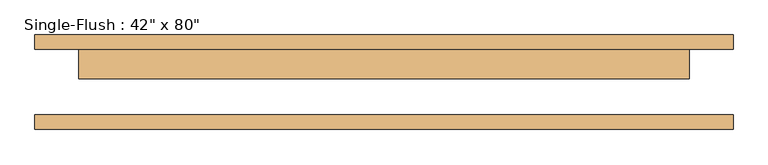
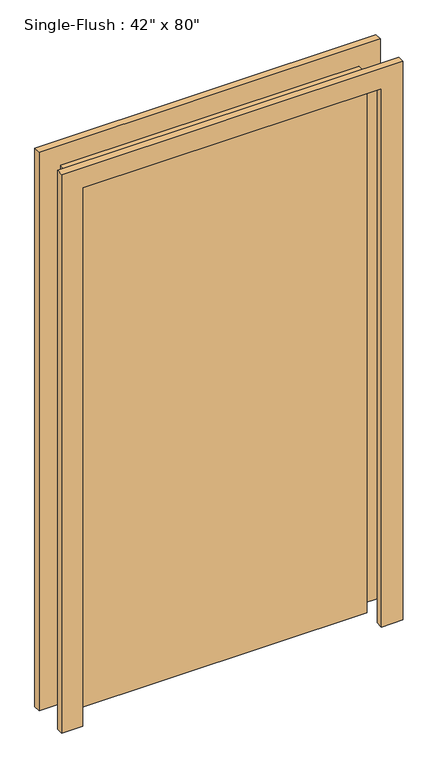
"""IFC4 building model written with IfcOpenShell, lengths in millimetres: door geometry."""

from ifc_helpers import new_model, si_unit, frame, origin, origin_with_axes, place, context, project, spatial, polyline, outline, extrude, source, transform, mapped, element, save


def door_5f0ed9dd(model_context):
    return source(origin(), model_context, "Body", "SweptSolid", [
        extrude(outline(polyline([(2108.2, -609.6), (0.0, -609.6), (0.0, -533.4), (2032.0, -533.4), (2032.0, 533.4), (0.0, 533.4), (0.0, 609.6), (2108.2, 609.6), (2108.2, -609.6)])), frame((0.0, 57.15, 0.0), z_axis=(0.0, 1.0, 0.0), x_axis=(0.0, 0.0, 1.0)), (0.0, 0.0, 1.0), 25.4),
        extrude(outline(polyline([(2108.2, 609.6), (2108.2, -609.6), (0.0, -609.6), (0.0, -533.4), (2032.0, -533.4), (2032.0, 533.4), (0.0, 533.4), (0.0, 609.6), (2108.2, 609.6)])), frame((0.0, -82.55, 0.0), z_axis=(0.0, 1.0, 0.0), x_axis=(0.0, 0.0, 1.0)), (0.0, 0.0, 1.0), 25.4),
        extrude(outline(polyline([(533.4, 6.35), (-533.4, 6.35), (-533.4, 57.15), (533.4, 57.15), (533.4, 6.35)])), origin_with_axes(), (0.0, 0.0, 1.0), 2032.0),
    ])


if __name__ == "__main__":
    model = new_model("IFC4")
    model_context = context("Model", 3, world=origin())
    ifc_project = project(units=[si_unit("LENGTHUNIT", "METRE", prefix="MILLI")], contexts=[model_context])
    site = spatial("IfcSite", under=ifc_project)
    building = spatial("IfcBuilding", under=site)
    placement = place(None, origin())
    door_shape = door_5f0ed9dd(model_context)
    element("IfcDoor", 1, ObjectType="Single-Flush : 42\" x 80\"", at=placement, inside=building, context=model_context, shape_type="MappedRepresentation", body=[
        mapped(door_shape, transform((0.0, 0.0, 0.0), x_axis=(1.0, 0.0, 0.0), y_axis=(0.0, 1.0, 0.0), z_axis=(0.0, 0.0, 1.0))),
    ])
    save(model, "model.ifc")

# Revit data of these elements
# Type "Single-Flush : 42\" x 80\""
#   Type Mark = "15"
#   Construction Type Id = "MDOOR"
#   Assembly Code = "C1020"
#   Analytic Construction = "Metal"
#   Thickness = 0' - 2"
#   Heat Transfer Coefficient (U) = 0.651978 BTU/(h·ft²·°F)
#   Height = 6' - 8"
#   Trim Projection Ext = 0' - 1"
#   Trim Projection Int = 0' - 1"
#   Trim Width = 0' - 3"
#   Width = 3' - 6"
#   Define Thermal Properties by = 1
#   Door Material = Door - Panel
#   Frame Material = Door - Frame
#   Visual Light Transmittance = 0
#   Solar Heat Gain Coefficient = 0
#   Function = (empty or 0)
#   Wall Closure = (empty or 0)
# Element 1 (IfcDoor, "Single-Flush : 42\" x 80\"")
#   Materials on its faces: "Door - Frame", "Door - Panel"
# Materials
#   "Door - Panel": class "Wood", colour RGB 210 159 95, transparency 0, Cost = 0
#   "Door - Frame": colour RGB 118 70 51, transparency 0, Cost = 0
